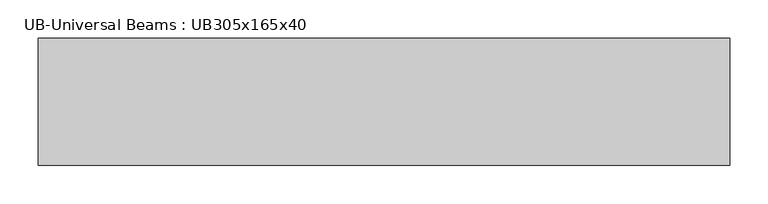
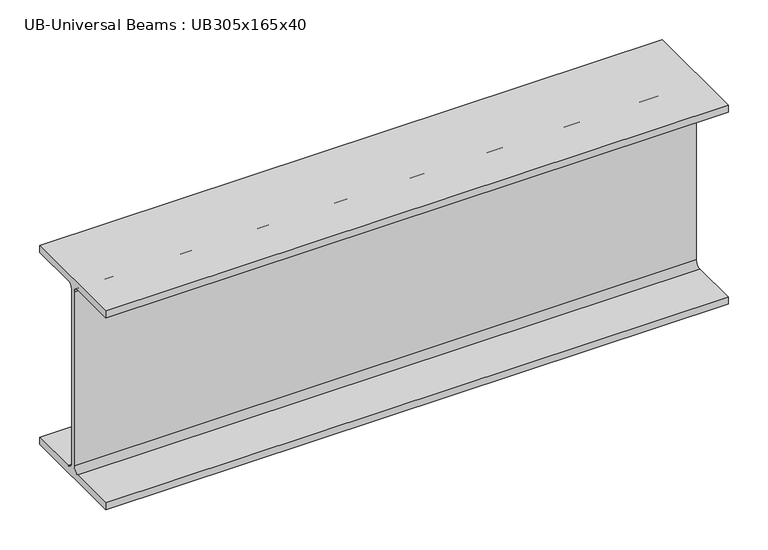
"""IFC4 building model written with IfcOpenShell, lengths in millimetres: beam geometry, UB-Universal Beams : UB305x165x40."""

from ifc_helpers import new_model, si_unit, point, frame, frame_2d, origin, place, context, project, spatial, polyline, circle_curve, trimmed, segment, composite_curve, outline, extrude, source, transform, mapped, element, save


def ub_universal_beams_ub305x165x40_e6c5e72d(model_context):
    return source(origin(), model_context, "Body", "SweptSolid", [
        extrude(outline(composite_curve([segment(polyline([(82.5, -141.5), (82.5, -151.7), (-82.5, -151.7), (-82.5, -141.5), (-11.9, -141.5)]), True, "CONTINUOUS"), segment(trimmed(circle_curve(frame_2d((-11.9, -132.6)), 8.9), [point((-11.9, -141.5))], [point((-3.0, -132.6))], True, "CARTESIAN"), True, "CONTINUOUS"), segment(polyline([(-3.0, -132.6), (-3.0, 132.6)]), True, "CONTINUOUS"), segment(trimmed(circle_curve(frame_2d((-11.9, 132.6)), 8.9), [point((-3.0, 132.6))], [point((-11.9, 141.5))], True, "CARTESIAN"), True, "CONTINUOUS"), segment(polyline([(-11.9, 141.5), (-82.5, 141.5), (-82.5, 151.7), (82.5, 151.7), (82.5, 141.5), (11.9, 141.5)]), True, "CONTINUOUS"), segment(trimmed(circle_curve(frame_2d((11.9, 132.6)), 8.9), [point((11.9, 141.5))], [point((3.0, 132.6))], True, "CARTESIAN"), True, "CONTINUOUS"), segment(polyline([(3.0, 132.6), (3.0, -132.6)]), True, "CONTINUOUS"), segment(trimmed(circle_curve(frame_2d((11.9, -132.6)), 8.9), [point((3.0, -132.6))], [point((11.9, -141.5))], True, "CARTESIAN"), True, "CONTINUOUS"), segment(polyline([(11.9, -141.5), (82.5, -141.5)]), True, "CONTINUOUS")], self_intersect=False)), frame((-460.6, 0.0, 0.0), z_axis=(1.0, 0.0, 0.0), x_axis=(0.0, 1.0, 0.0)), (0.0, 0.0, 1.0), 899.0),
    ])


if __name__ == "__main__":
    model = new_model("IFC4")
    model_context = context("Model", 3, world=origin())
    ifc_project = project(units=[si_unit("LENGTHUNIT", "METRE", prefix="MILLI")], contexts=[model_context])
    site = spatial("IfcSite", under=ifc_project)
    building = spatial("IfcBuilding", under=site)
    placement = place(None, origin())
    ub_universal_beams_ub305x165x40_shape = ub_universal_beams_ub305x165x40_e6c5e72d(model_context)
    element("IfcBeam", 1, ObjectType="UB-Universal Beams : UB305x165x40", at=placement, inside=building, context=model_context, shape_type="MappedRepresentation", body=[
        mapped(ub_universal_beams_ub305x165x40_shape, transform((0.0, 0.0, 0.0), x_axis=(1.0, 0.0, 0.0), y_axis=(0.0, 1.0, 0.0), z_axis=(0.0, 0.0, 1.0))),
    ])
    save(model, "model.ifc")

# Revit data of these elements
# Type "UB-Universal Beams : UB305x165x40"
#   Section Name Key = "UB305X165X40"
#   Width = 16.5 cm
#   Web Thickness = 0.6 cm
#   Web Fillet = 0.89 cm
#   Warping Constant = 164000.0 cm⁶
#   Torsional Moment of Inertia = 14.70 cm⁴
#   Section Area = 51.3 cm²
#   Plastic Modulus weak axis = 142.0 cm³
#   Plastic Modulus strong axis = 623.0 cm³
#   Nominal Weight = 40.2999 kgf/m
#   Moment of Inertia weak axis = 764.00 cm⁴
#   Moment of Inertia strong axis = 8503.00 cm⁴
#   Height = 30.34 cm
#   Flange Thickness = 1.02 cm
#   Elastic Modulus weak axis = 92.6 cm³
#   Elastic Modulus strong axis = 560.0 cm³
#   Centroid Vertical = 15.17 cm
#   Centroid Horizontal = 8.25 cm
#   Bolt Spacing = 9.0 cm
#   Length [instance default] = 1500 mm
#   Structural Material [instance default] = Metal - Steel 43-275
#   Type Comments = ""
#   Assembly Code = ""
# Element 1 (IfcBeam, "UB-Universal Beams : UB305x165x40")
#   Materials on its faces: "Metal - Steel 43-275"
# Materials
#   "Metal - Steel 43-275": class "Metal", colour RGB 247 247 247, transparency 0, Cost = 0
